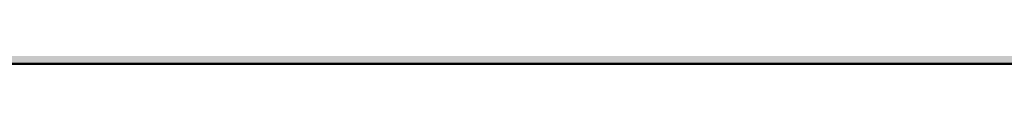
# Model space of a CAD drawing. Units: millimetres. Extents: x 0 to 2267, y 0 to 1823.
# Tile 252 of 256: x 1843.095 to 1843.2685, y 1127.4171 to 1127.4171. Entities that reach past the tile are written whole.
import ezdxf

# ---------------------------------------------------------------- set-up
doc = ezdxf.new("R2010")
doc.units = ezdxf.units.MM
doc.header["$MEASUREMENT"] = 0
for name, color, linetype, lineweight in [('M-DIMS', 2, 'Continuous', 25), ('M-HATC', 252, 'Continuous', 18), ('M-OUTL', 7, 'Continuous', 50)]:
    doc.layers.add(name, color=color, linetype=linetype, lineweight=lineweight)
doc.styles.get("Standard").update_dxf_attribs({"font": 'arial.ttf'})
doc.dimstyles.get("Standard").update_dxf_attribs({"dimtxt": 7, "dimasz": 4, "dimexe": 0.18, "dimexo": 0.0625, "dimgap": 0.09, "dimtad": 0, "dimdec": 0, "dimzin": 0, "dimdsep": 46, "dimtxsty": 'Standard', "dimcen": 0.09, "dimadec": 0, "dimazin": 0, "dimtfac": 1, "dimtdec": 0, "dimtofl": 0, "dimtmove": 0, "dimatfit": 3, "dimfxl": 1, "dimtolj": 1, "dimtzin": 0, "dimarcsym": 0})

# ---------------------------------------------------------------- blocks, each defined once
blk = doc.blocks.new('*D1')
at = {"layer": 'Defpoints', "color": 0, "transparency": 16777216}
for p in [(1593.42891, 1127.41706), (1843.42891, 1127.41706), (1843.42891, 955.62775)]:
    blk.add_point(p, dxfattribs=at)
at = {"layer": 'M-DIMS', "color": 0, "lineweight": -2, "transparency": 16777216}
for p, q in [((1593.42891, 1127.35456), (1593.42891, 955.44775)), ((1843.42891, 1127.35456), (1843.42891, 955.44775)), ((1597.42891, 955.62775), (1710.55821, 955.62775)), ((1839.42891, 955.62775), (1726.2996, 955.62775))]:
    blk.add_line(p, q, dxfattribs=at)
at = {"layer": 'M-DIMS', "color": 0, "transparency": 16777216}
for points in [[(1597.42891, 956.29442), (1597.42891, 954.96109), (1593.42891, 955.62775)], [(1839.42891, 956.29442), (1839.42891, 954.96109), (1843.42891, 955.62775)]]:
    blk.add_solid(points, dxfattribs=at)
at = {"layer": 'M-DIMS', "color": 0, "transparency": 16777216, "insert": (1718.42891, 955.62775), "char_height": 7, "attachment_point": 5}
blk.add_mtext('\\A1;250', dxfattribs=at)

msp = doc.modelspace()

# ---------------------------------------------------------------- hatches: boundary and pattern name
at = {"layer": 'M-HATC'}
h = msp.add_hatch(color=256, dxfattribs=at)
h.dxf.hatch_style = 1
h.paths.add_polyline_path([(2042.88863, 1580.17963), (2055.77105, 1593.06204), (1381.08677, 1593.06204), (1393.96918, 1580.17963), (1374.08597, 1560.29642), (2062.77184, 1560.29642)])
h.paths.add_polyline_path([(1843.42891, 1201.32971), (1843.42891, 1227.24746), (1593.42891, 1227.24746), (1593.42891, 1201.32971, -0.228274), (1574.59893, 1162.23457), (1530.92891, 1127.41706), (1905.92891, 1127.41706), (1862.25888, 1162.23457, -0.228274)])

# ---------------------------------------------------------------- linework, layer by layer
at = {"layer": 'M-OUTL'}
msp.add_line((1530.92891, 1127.41706), (1905.92891, 1127.41706), dxfattribs=at)

# ---------------------------------------------------------------- dimensions: what is measured, and where the dimension line sits
at = {"layer": 'M-DIMS'}
dim = msp.add_linear_dim(base=(1843.42891, 955.62775), p1=(1593.42891, 1127.41706), p2=(1843.42891, 1127.41706), dimstyle='Standard', override={"dimclrd": 0, "dimclre": 0, "dimclrt": 0}, dxfattribs=at)
dim.commit()
dim.dimension.update_dxf_attribs({"geometry": '*D1', "text_midpoint": (1718.42891, 955.62775)})

doc.saveas('drawing.dxf')
